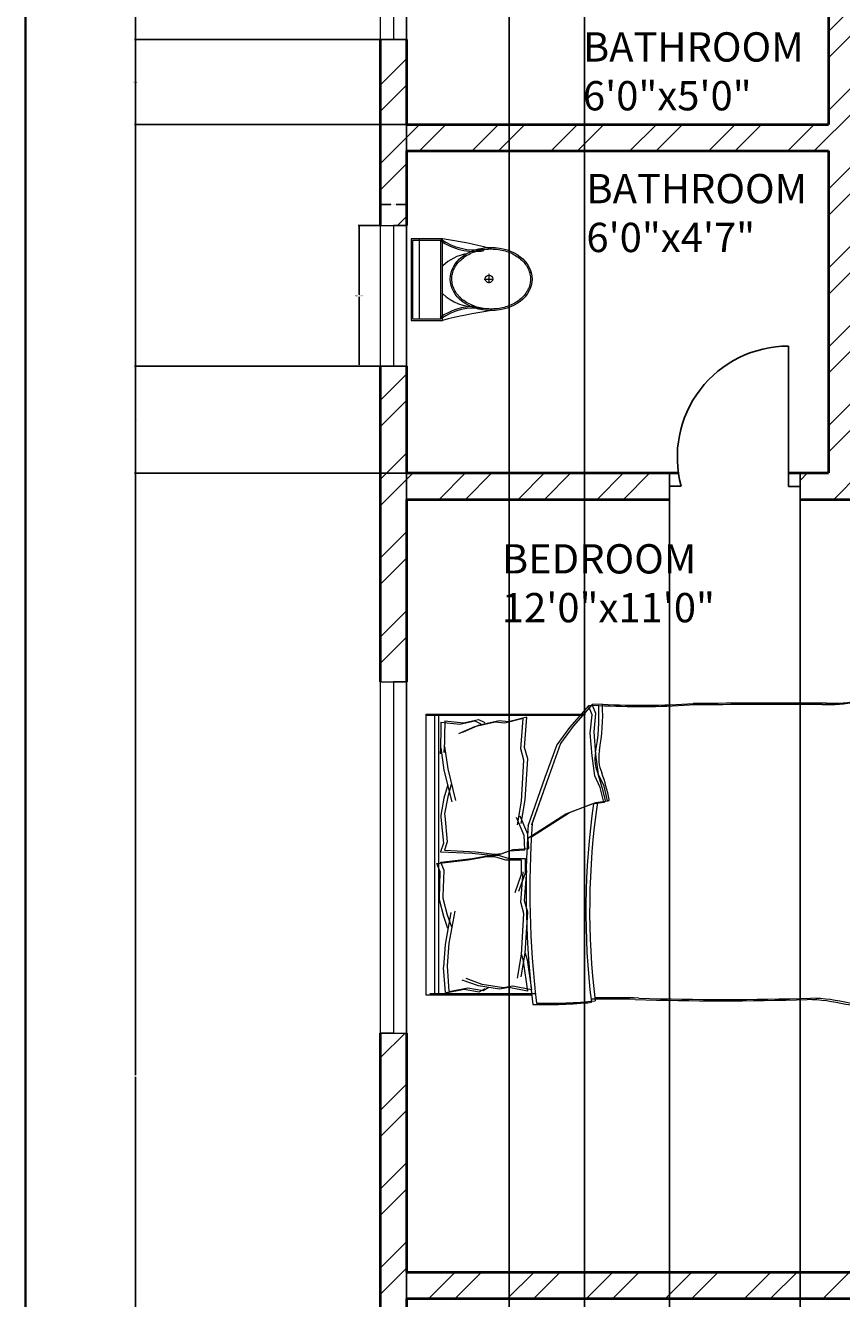
# Model space of a CAD drawing. Units: inches. Extents: x 2063 to 2617, y 1299 to 2210.
# Tile 6 of 22: x 2063 to 2202, y 1727 to 1945. Entities that reach past the tile are written whole.
import ezdxf

# ---------------------------------------------------------------- set-up
doc = ezdxf.new("R2010")
doc.units = ezdxf.units.IN
for name, color, linetype, lineweight in [('A-ANNO-DIMS', 2, 'Continuous', 18), ('A-ANNO-TTLB', 7, 'Continuous', 35), ('A-AREA-IDEN', 7, 'Continuous', 18), ('A-DOOR', 11, 'Continuous', 25), ('A-FLOR-FIXT', 8, 'Continuous', 18), ('A-FURN', 8, 'Continuous', 18), ('A-GLAZ', 123, 'Continuous', 18), ('A-WALL', 7, 'Continuous', 40)]:
    doc.layers.add(name, color=color, linetype=linetype, lineweight=lineweight)
doc.layers.add('A-WALL-PATT', color=215, linetype='Continuous', lineweight=13, true_color=0xa953a0)
doc.styles.get("Standard").update_dxf_attribs({"font": 'arial.ttf'})
doc.dimstyles.get("Standard").update_dxf_attribs({"dimtxt": 0.18, "dimasz": 0.18, "dimexe": 0.18, "dimexo": 0.0625, "dimgap": 0.09, "dimtad": 0, "dimtih": 1, "dimtoh": 1, "dimdec": 4, "dimzin": 0, "dimdsep": 46, "dimtxsty": 'Standard', "dimcen": 0.09, "dimadec": 0, "dimazin": 0, "dimtfac": 1, "dimtdec": 4, "dimtofl": 0, "dimtmove": 0, "dimatfit": 3, "dimfxl": 1, "dimtolj": 1, "dimtzin": 0, "dimarcsym": 0})

# ---------------------------------------------------------------- blocks, each defined once
blk = doc.blocks.new('A$C31115884')
for p, q in [((283.1, 497.7), (223.4, 497.7)), ((257.5, 466.4), (257.5, 523.2)), ((0, 200), (0, 0)), ((520, 200), (0, 200)), ((10, 190), (10, 10)), ((510, 190), (10, 190)), ((510, 10), (510, 190)), ((520, 0), (520, 200)), ((510, 54.5), (0, 54.5)), ((10, 10), (510, 10)), ((0, 0), (520, 0))]:
    blk.add_line(p, q)
blk.add_circle((255.6, 496.4), 23.6)
for centre, radius, start, end in [((2777.7, -204.6), 2807, 165.4549, 171.71327), ((3237, 905), 2807, 188.28673, 194.5451), ((-294.5, 403.3), 364.7, 324.20913, 9.34987), ((-294.5, 403.3), 374.7, 324.20913, 9.34987), ((139.5, 406.2), 293.5, 315.84364, 2.65635), ((805.8, 403.3), 374.7, 179.20365, 215.79087), ((805.8, 403.3), 364.7, 170.65013, 215.79087), ((383.6, 406.2), 293.5, 190.27735, 224.15636)]:
    blk.add_arc(centre, radius, start, end)
blk.add_ellipse((256.2, 509.9), major_axis=(0, -260.7), ratio=0.772727)
blk.add_open_spline([(256.2, 259.2), (263.1, 259.2), (270, 259.7), (287.8, 262.3), (298.7, 265.1), (319.9, 273.1), (330.2, 278.4), (350.1, 291.1), (359.7, 298.7), (377.7, 315.9), (386.2, 325.5), (401.7, 346.6), (408.8, 358.1), (421.3, 382.5), (426.8, 395.5), (435.9, 422.4), (439.5, 436.4), (444.8, 465.1), (446.5, 479.7), (447.9, 509.2), (447.6, 524), (445, 553.3), (442.7, 567.8), (436.3, 596), (432.1, 609.7), (421.9, 636), (416, 648.6), (402.5, 672.1), (395, 683), (378.6, 703), (369.8, 712.1), (351.1, 728), (341.3, 734.8), (320.9, 746.2), (310.4, 750.7), (288.9, 757.3), (278, 759.4), (256, 761), (245, 760.6), (223.1, 757.2), (212.3, 754.3), (191.1, 746.1), (180.8, 740.7), (160.9, 727.8), (151.4, 720.1), (133.5, 702.7), (125.1, 693), (109.6, 671.7), (102.6, 660.2), (90.2, 635.7), (84.9, 622.7), (76, 595.6), (72.4, 581.6), (67.2, 552.9), (65.6, 538.2), (64.4, 508.8), (64.8, 494), (67.5, 464.7), (69.9, 450.2), (76.6, 422), (80.8, 408.3), (91.1, 382.2), (97.2, 369.7), (110.8, 346.3), (118.4, 335.4), (134.8, 315.6), (143.7, 306.7), (162.4, 290.9), (172.3, 284.2), (192.8, 273), (203.3, 268.6), (224.8, 262.2), (235.8, 260.2), (249.9, 259.3), (253, 259.2), (256.2, 259.2)], degree=3, knots=[0, 0, 0, 0, 0.110105, 0.110105, 0.285049, 0.285049, 0.459994, 0.459994, 0.634938, 0.634938, 0.809882, 0.809882, 0.984827, 0.984827, 1.159771, 1.159771, 1.334715, 1.334715, 1.50966, 1.50966, 1.684604, 1.684604, 1.859549, 1.859549, 2.034493, 2.034493, 2.209437, 2.209437, 2.384382, 2.384382, 2.559326, 2.559326, 2.73427, 2.73427, 2.909215, 2.909215, 3.084159, 3.084159, 3.259103, 3.259103, 3.434048, 3.434048, 3.608992, 3.608992, 3.783936, 3.783936, 3.958881, 3.958881, 4.133825, 4.133825, 4.30877, 4.30877, 4.483714, 4.483714, 4.658658, 4.658658, 4.833603, 4.833603, 5.008547, 5.008547, 5.183491, 5.183491, 5.358436, 5.358436, 5.53338, 5.53338, 5.708324, 5.708324, 5.883269, 5.883269, 6.058213, 6.058213, 6.233158, 6.233158, 6.283185, 6.283185, 6.283185, 6.283185])
blk = doc.blocks.new('BED-DOUBLE')
for p, q in [((3.48, 63.33), (3.48, 81.44)), ((3.48, 63.33), (3.48, 81.44)), ((3.48, 81.44), (51.49, 81.44)), ((3.7, 62.69), (3.7, 80.8)), ((3.7, 62.69), (3.7, 80.8)), ((51.27, 81.44), (51.27, 54.83)), ((51.27, 81.44), (51.27, 54.83)), ((51.49, 81.44), (51.49, 80.8)), ((51.49, 80.8), (51.49, 54.19)), ((51.49, 80.8), (51.49, 54.19)), ((3.48, 79.91), (51.27, 79.91)), ((3.48, 79.91), (51.27, 79.91)), ((3.7, 79.27), (51.49, 79.27)), ((3.7, 79.27), (51.49, 79.27)), ((3.9, 78.11), (8.18, 78.43)), ((3.9, 78.11), (8.18, 78.43)), ((8.18, 78.43), (8.29, 78.42)), ((8.18, 78.43), (8.29, 78.42)), ((8.29, 78.42), (12.11, 78.13)), ((8.29, 78.42), (12.11, 78.13)), ((14.86, 77.69), (16.88, 78.42)), ((14.86, 77.69), (16.88, 78.42)), ((16.88, 78.42), (19.77, 79.14)), ((16.88, 78.42), (19.77, 79.14)), ((17.11, 77.78), (20, 78.5)), ((17.11, 77.78), (20, 78.5)), ((19.77, 79.14), (20.09, 79.14)), ((19.77, 79.14), (20.09, 79.14)), ((20, 78.5), (20.32, 78.5)), ((20, 78.5), (20.32, 78.5)), ((20.09, 79.14), (24.54, 79)), ((20.09, 79.14), (24.54, 79)), ((20.32, 78.5), (24.77, 78.36)), ((20.32, 78.5), (24.77, 78.36)), ((24.54, 79), (25.98, 79.57)), ((24.54, 79), (25.98, 79.57)), ((24.77, 78.36), (26.21, 78.93)), ((24.77, 78.36), (26.21, 78.93)), ((25.98, 79.57), (26.56, 74.22)), ((25.98, 79.57), (26.56, 74.22)), ((26.21, 78.93), (26.79, 73.58)), ((26.21, 78.93), (26.79, 73.58)), ((27.98, 78.95), (27.73, 73.58)), ((27.98, 78.95), (27.73, 73.58)), ((28.21, 78.31), (27.96, 72.94)), ((28.21, 78.31), (27.96, 72.94)), ((29.46, 78.46), (27.98, 78.95)), ((29.46, 78.46), (27.98, 78.95)), ((29.68, 77.83), (28.21, 78.31)), ((29.68, 77.83), (28.21, 78.31)), ((33.88, 78.89), (29.46, 78.46)), ((33.88, 78.89), (29.46, 78.46)), ((34.21, 78.91), (33.88, 78.89)), ((34.2, 78.91), (33.88, 78.89)), ((37.14, 78.37), (34.2, 78.91)), ((37.14, 78.37), (34.21, 78.91)), ((41.91, 78.37), (36.5, 77.02)), ((41.91, 78.37), (36.5, 77.02)), ((39.2, 77.77), (37.14, 78.37)), ((39.2, 77.77), (37.14, 78.37)), ((45.71, 78.9), (41.91, 78.37)), ((45.71, 78.9), (41.91, 78.37)), ((50.11, 78.89), (44.71, 78.98)), ((44.71, 78.98), (45.71, 78.9)), ((50.11, 78.89), (44.71, 78.98)), ((44.71, 78.98), (45.71, 78.9)), ((50.34, 78.25), (44.94, 78.34)), ((44.94, 78.34), (45.94, 78.26)), ((50.34, 78.25), (44.94, 78.34)), ((44.94, 78.34), (45.94, 78.26)), ((50.11, 78.89), (49.73, 75.68)), ((50.11, 78.89), (49.73, 75.68)), ((3.89, 78.13), (4.47, 74.95)), ((3.9, 78.13), (4.47, 74.95)), ((4.12, 77.49), (4.7, 74.31)), ((4.12, 77.49), (4.7, 74.31)), ((4.13, 77.47), (8.41, 77.8)), ((4.13, 77.47), (8.41, 77.8)), ((8.41, 77.8), (8.51, 77.78)), ((8.41, 77.8), (8.51, 77.78)), ((8.51, 77.78), (12.34, 77.49)), ((8.51, 77.78), (12.34, 77.49)), ((12.11, 78.13), (17.6, 77.12)), ((12.11, 78.13), (17.6, 77.12)), ((12.34, 77.49), (17.83, 76.48)), ((12.34, 77.49), (17.83, 76.48)), ((15.08, 77.05), (17.11, 77.78)), ((15.08, 77.05), (17.11, 77.78)), ((34.11, 78.25), (29.68, 77.83)), ((34.11, 78.25), (29.68, 77.83)), ((34.43, 78.27), (34.11, 78.25)), ((34.43, 78.27), (34.11, 78.25)), ((37.36, 77.73), (34.43, 78.27)), ((37.36, 77.73), (34.43, 78.27)), ((42.14, 77.73), (36.72, 76.38)), ((42.14, 77.73), (36.72, 76.38)), ((39.43, 77.13), (37.36, 77.73)), ((39.43, 77.13), (37.36, 77.73)), ((45.94, 78.26), (42.14, 77.73)), ((45.94, 78.26), (42.14, 77.73)), ((50.34, 78.25), (49.96, 75.04)), ((50.34, 78.25), (49.96, 75.04)), ((4.47, 74.95), (4.04, 72.34)), ((4.47, 74.95), (4.04, 72.34)), ((4.7, 74.31), (4.27, 71.7)), ((4.7, 74.31), (4.27, 71.7)), ((5.05, 72.49), (6.06, 75.24)), ((5.05, 72.49), (6.06, 75.24)), ((5.28, 71.85), (6.29, 74.6)), ((5.28, 71.85), (6.29, 74.6)), ((26.56, 74.22), (27.14, 71.04)), ((26.56, 74.22), (27.14, 71.04)), ((49.31, 73.19), (48.13, 75.87)), ((49.31, 73.19), (48.13, 75.87)), ((49.54, 72.55), (48.36, 75.23)), ((49.54, 72.55), (48.36, 75.23)), ((49.73, 75.68), (50.33, 73.11)), ((49.73, 75.68), (50.33, 73.11)), ((49.96, 75.04), (50.56, 72.47)), ((49.96, 75.04), (50.56, 72.47)), ((4.04, 72.34), (4.62, 71.33)), ((4.04, 72.34), (4.62, 71.33)), ((4.47, 68.87), (5.05, 72.49)), ((4.47, 68.87), (5.05, 72.49)), ((4.7, 68.23), (5.28, 71.85)), ((4.7, 68.23), (5.28, 71.85)), ((26.79, 73.58), (27.37, 70.4)), ((26.79, 73.58), (27.37, 70.4)), ((27.73, 73.58), (27.36, 70.37)), ((27.73, 73.58), (27.36, 70.37)), ((27.96, 72.94), (27.58, 69.73)), ((27.96, 72.94), (27.58, 69.73)), ((50.11, 69.61), (49.31, 73.19)), ((50.11, 69.61), (49.31, 73.19)), ((50.34, 68.98), (49.54, 72.55)), ((50.34, 68.98), (49.54, 72.55)), ((50.33, 73.11), (49.81, 72.06)), ((50.33, 73.11), (49.82, 72.06)), ((50.56, 72.47), (50.04, 71.42)), ((50.56, 72.47), (50.04, 71.42)), ((4.27, 71.7), (4.85, 70.69)), ((4.27, 71.7), (4.85, 70.69)), ((27.14, 69.74), (26.56, 67.86)), ((27.14, 69.74), (26.56, 67.86)), ((27.14, 71.04), (27.14, 69.74)), ((27.14, 71.04), (27.14, 69.74)), ((27.36, 70.37), (27.44, 69.07)), ((27.36, 70.37), (27.44, 69.07)), ((27.37, 70.4), (27.37, 69.1)), ((27.37, 70.4), (27.37, 69.1)), ((27.58, 69.73), (27.66, 68.43)), ((27.58, 69.73), (27.66, 68.43)), ((49.92, 68.01), (50.11, 69.61)), ((49.92, 68.01), (50.11, 69.61)), ((4.76, 67.28), (4.47, 68.87)), ((4.76, 67.28), (4.47, 68.87)), ((4.99, 66.64), (4.7, 68.23)), ((4.99, 66.64), (4.7, 68.23)), ((26.56, 67.86), (26.56, 65.18)), ((26.56, 67.86), (26.56, 65.18)), ((27.37, 69.1), (26.79, 67.22)), ((27.37, 69.1), (26.79, 67.22)), ((27.44, 69.07), (28.13, 67.23)), ((27.44, 69.07), (28.13, 67.23)), ((27.66, 68.43), (28.36, 66.59)), ((27.66, 68.43), (28.36, 66.59)), ((50.7, 64.87), (49.92, 68.01)), ((50.7, 64.87), (49.92, 68.01)), ((50.15, 67.37), (50.34, 68.98)), ((50.15, 67.37), (50.34, 68.98)), ((4.18, 64.1), (4.76, 67.28)), ((4.18, 64.1), (4.76, 67.28)), ((4.41, 63.46), (4.99, 66.64)), ((4.41, 63.46), (4.99, 66.64)), ((6.38, 65.82), (10.41, 65.15)), ((6.38, 65.82), (10.41, 65.15)), ((17.42, 64.72), (19.38, 65.27)), ((17.42, 64.72), (19.38, 65.27)), ((19.38, 65.27), (24.52, 64.87)), ((19.38, 65.27), (24.52, 64.87)), ((24.1, 65.18), (20.96, 66.27)), ((24.1, 65.18), (20.96, 66.27)), ((24.33, 64.54), (21.19, 65.63)), ((24.33, 64.54), (21.19, 65.63)), ((26.79, 67.22), (26.79, 64.54)), ((26.79, 67.22), (26.79, 64.54)), ((28.13, 67.23), (28.3, 64.55)), ((28.13, 67.23), (28.3, 64.55)), ((28.36, 66.59), (28.53, 63.91)), ((28.36, 66.59), (28.53, 63.91)), ((30.75, 64.7), (33.82, 65.99)), ((30.75, 64.7), (33.82, 65.99)), ((30.98, 64.06), (34.05, 65.35)), ((30.98, 64.06), (34.05, 65.35)), ((32.56, 65.82), (36.6, 65.15)), ((32.56, 65.82), (36.6, 65.15)), ((43.61, 64.72), (45.57, 65.27)), ((43.61, 64.72), (45.57, 65.27)), ((45.57, 65.27), (50.7, 64.87)), ((45.57, 65.27), (50.7, 64.87)), ((50.93, 64.23), (50.15, 67.37)), ((50.93, 64.23), (50.15, 67.37)), ((9.28, 64.83), (4.18, 64.1)), ((9.28, 64.83), (4.18, 64.1)), ((9.51, 64.19), (4.41, 63.46)), ((9.51, 64.19), (4.41, 63.46)), ((6.61, 65.18), (10.64, 64.51)), ((6.61, 65.18), (10.64, 64.51)), ((10.41, 65.15), (9.28, 64.83)), ((10.41, 65.15), (9.28, 64.83)), ((10.64, 64.51), (9.51, 64.19)), ((10.64, 64.51), (9.51, 64.19)), ((10.41, 65.15), (17.42, 64.72)), ((10.41, 65.15), (17.42, 64.72)), ((10.64, 64.51), (17.65, 64.08)), ((10.64, 64.51), (17.65, 64.08)), ((17.65, 64.08), (19.61, 64.64)), ((17.65, 64.08), (19.61, 64.64)), ((19.61, 64.64), (24.74, 64.23)), ((19.61, 64.64), (24.74, 64.23)), ((26.56, 65.18), (24.1, 65.18)), ((26.56, 65.18), (24.1, 65.18)), ((26.79, 64.54), (24.33, 64.54)), ((26.79, 64.54), (24.33, 64.54)), ((28.3, 64.55), (30.75, 64.7)), ((28.3, 64.55), (30.75, 64.7)), ((28.53, 63.91), (30.98, 64.06)), ((28.53, 63.91), (30.98, 64.06)), ((30.26, 64.06), (34.45, 57.57)), ((30.26, 64.06), (34.45, 57.57)), ((30.49, 63.42), (34.68, 56.93)), ((30.49, 63.42), (34.68, 56.93)), ((40.64, 61.13), (32.31, 64.06)), ((40.64, 61.13), (32.31, 64.06)), ((40.87, 60.49), (32.53, 63.42)), ((40.87, 60.49), (32.54, 63.42)), ((32.79, 65.18), (36.83, 64.51)), ((32.79, 65.18), (36.82, 64.51)), ((36.6, 65.15), (43.61, 64.72)), ((36.6, 65.15), (43.61, 64.72)), ((36.82, 64.51), (43.83, 64.08)), ((36.83, 64.51), (43.84, 64.08)), ((43.83, 64.08), (45.8, 64.64)), ((43.84, 64.08), (45.8, 64.64)), ((45.8, 64.64), (50.93, 64.23)), ((45.8, 64.64), (50.93, 64.23)), ((46.22, 59.11), (40.64, 61.13)), ((46.22, 59.11), (40.64, 61.13)), ((46.45, 58.48), (40.87, 60.49)), ((46.45, 58.48), (40.87, 60.49)), ((49.16, 56.95), (46.22, 59.11)), ((49.16, 56.95), (46.22, 59.11)), ((34.45, 57.57), (36.15, 53.08)), ((34.45, 57.57), (36.15, 53.08)), ((34.68, 56.93), (36.38, 52.44)), ((34.68, 56.93), (36.38, 52.44)), ((49.39, 56.31), (46.45, 58.48)), ((49.39, 56.31), (46.45, 58.48)), ((52.87, 53.7), (49.16, 56.95)), ((52.87, 53.7), (49.16, 56.95)), ((53.1, 53.06), (49.39, 56.31)), ((53.1, 53.06), (49.39, 56.31)), ((36.15, 53.08), (36.46, 51.07)), ((36.15, 53.08), (36.46, 51.07)), ((36.38, 52.44), (36.69, 50.43)), ((36.38, 52.44), (36.69, 50.43)), ((38.94, 51.69), (40.95, 52.61)), ((38.94, 51.69), (40.95, 52.61)), ((40.95, 52.61), (44.36, 53.08)), ((40.95, 52.61), (44.36, 53.08)), ((41.18, 51.97), (44.59, 52.44)), ((41.18, 51.97), (44.59, 52.44)), ((44.36, 53.08), (48.23, 53.39)), ((44.36, 53.08), (48.23, 53.39)), ((44.59, 52.44), (48.46, 52.75)), ((44.59, 52.44), (48.46, 52.75)), ((48.23, 53.39), (51.33, 53.08)), ((48.23, 53.39), (51.33, 53.08)), ((48.46, 52.75), (51.56, 52.44)), ((48.46, 52.75), (51.56, 52.44)), ((51.33, 53.08), (52.87, 53.7)), ((51.33, 53.08), (52.87, 53.7)), ((51.56, 52.44), (53.1, 53.06)), ((51.56, 52.44), (53.1, 53.06)), ((52.95, 51.95), (52.87, 53.7, 3.87)), ((52.95, 51.95), (52.87, 53.7, 3.87)), ((53.18, 51.31), (53.1, 53.06, 3.87)), ((53.18, 51.31), (53.1, 53.06, 3.87)), ((36.46, 51.07), (38.94, 51.69)), ((36.46, 51.07), (38.94, 51.69)), ((36.69, 50.43), (39.17, 51.05)), ((36.69, 50.43), (39.17, 51.05)), ((39.17, 51.05), (41.18, 51.97)), ((39.17, 51.05), (41.18, 51.97)), ((15.06, 2.2), (39.68, 2.2)), ((15.06, 2.2), (39.68, 2.2)), ((15.29, 1.56), (39.91, 1.56)), ((15.29, 1.56), (39.91, 1.56))]:
    blk.add_line(p, q)
for centre, radius, start, end in [((85.16, 61.35), 83.31, 178.7218, 185.604), ((85.16, 61.35), 83.31, 178.7218, 185.604), ((21.36, -100.61), 164.97, 86.0865, 96.7821), ((21.36, -100.61), 164.97, 86.0865, 96.7821), ((21.59, -101.25), 164.97, 86.0865, 96.7821), ((21.59, -101.25), 164.97, 86.0865, 96.7821), ((85.39, 60.71), 83.31, 178.7218, 185.604), ((85.39, 60.71), 83.31, 178.7218, 185.604), ((17.76, -74.87), 129.02, 81.7845, 96.9006), ((17.76, -74.87), 129.02, 81.7845, 96.9006), ((17.98, -75.51), 129.02, 81.7845, 96.9006), ((17.98, -75.51), 129.02, 81.7845, 96.9006), ((-167.31, 50.27), 170.11, 358.4762, 1.0082), ((-167.31, 50.27), 170.11, 358.4762, 1.0082), ((-167.08, 49.63), 170.11, 358.4762, 1.0082), ((-167.08, 49.63), 170.11, 358.4762, 1.0082), ((43.74, 46.38), 6.22, 78.6608, 113.7384), ((43.74, 46.38), 6.22, 78.6608, 113.7384), ((51.33, 88.1), 36.18, 259.8763, 272.5657), ((51.33, 88.1), 36.18, 259.8763, 272.5657), ((36.64, 51), 0.185, 160.2464, 271.1377), ((36.64, 51), 0.185, 160.2464, 271.1377), ((31.15, 79.96), 29.65, 280.6617, 289.8806), ((31.15, 79.96), 29.65, 280.6617, 289.8806), ((36.87, 50.36), 0.185, 160.2464, 271.1377), ((36.86, 50.36), 0.185, 160.2464, 271.1377), ((31.38, 79.32), 29.65, 280.6617, 289.8806), ((31.38, 79.32), 29.65, 280.6617, 289.8806), ((43.97, 45.74), 6.22, 78.6608, 113.7384), ((43.97, 45.74), 6.22, 78.6608, 113.7384), ((51.56, 87.46), 36.18, 259.8763, 272.5657), ((51.56, 87.46), 36.18, 259.8763, 272.5657), ((182.27, 45.13), 129.5, 176.9791, 183.8365), ((182.27, 45.13), 129.5, 176.9791, 183.8365), ((182.49, 44.49), 129.5, 176.9791, 183.8365), ((182.49, 44.49), 129.5, 176.9791, 183.8365), ((484.82, 30.83), 482.31, 178.2277, 181.7185), ((484.82, 30.83), 482.31, 178.2277, 181.7185), ((485.05, 30.19), 482.31, 178.2277, 181.7185), ((485.05, 30.19), 482.31, 178.2277, 181.7185), ((-4508.74, 13.62), 4561.86, 0.00217, 0.28689), ((-4508.74, 13.62), 4561.86, 0.00217, 0.28689), ((-4508.51, 12.98), 4561.86, 0.00217, 0.28689), ((-4508.51, 12.98), 4561.86, 0.00217, 0.28689), ((-26.9, 16.93), 29.63, 346.0648, 358.9113), ((-26.9, 16.93), 29.63, 346.0648, 358.9113), ((-26.67, 16.29), 29.63, 346.0648, 358.9113), ((-26.67, 16.29), 29.63, 346.0648, 358.9113), ((76.16, 12.78), 23.07, 177.4714, 206.4681), ((76.16, 12.78), 23.07, 177.4714, 206.4681), ((76.39, 12.14), 23.07, 177.4714, 206.4681), ((76.39, 12.14), 23.07, 177.4714, 206.4681), ((-21.66, 11.17), 23.56, 337.9751, 356.652), ((-21.66, 11.17), 23.56, 337.9751, 356.652), ((-21.43, 10.53), 23.56, 337.9751, 356.652), ((-21.43, 10.53), 23.56, 337.9751, 356.652), ((1.09, 1.73), 1.09, 146.1736, 293.4781), ((1.09, 1.73), 1.09, 146.1736, 293.4781), ((21.43, -119.39), 121.76, 92.9958, 99.4091), ((21.43, -119.39), 121.76, 92.9958, 99.4091), ((-17.22, 105.16), 106.46, 283.3832, 287.7053), ((-17.22, 105.16), 106.46, 283.3832, 287.7053), ((-16.99, 104.52), 106.46, 283.3832, 287.7053), ((-16.99, 104.52), 106.46, 283.3832, 287.7053), ((41.15, -130.83), 133.04, 84.4998, 90.6351), ((41.15, -130.83), 133.04, 84.4998, 90.6351), ((54.41, 2.57), 1.1, 242.6588, 356.02), ((54.41, 2.57), 1.1, 242.6588, 356.02), ((1.32, 1.09), 1.09, 146.1736, 293.4781), ((1.32, 1.09), 1.09, 146.1736, 293.4781), ((21.66, -120.03), 121.76, 92.9958, 99.4091), ((21.66, -120.03), 121.76, 92.9958, 99.4091), ((41.38, -131.47), 133.04, 84.4998, 90.6351), ((41.38, -131.47), 133.04, 84.4998, 90.6351), ((54.64, 1.93), 1.1, 242.6588, 356.02), ((54.64, 1.93), 1.1, 242.6588, 356.02)]:
    blk.add_arc(centre, radius, start, end)
blk = doc.blocks.new('WIN-60IN')
for p, q in [((0, 60), (4.5, 60)), ((0, 60), (0, 0)), ((4.5, 60), (2.25, 60)), ((2.25, 60), (2.25, 0)), ((4.5, 60), (4.5, 0)), ((2.25, 0), (0, 0)), ((0, 0), (4.5, 0))]:
    blk.add_line(p, q)
blk = doc.blocks.new('WIN-24IN')
for p, q in [((0, 24), (4.5, 24)), ((0, 24), (0, 0)), ((4.5, 24), (2.25, 24)), ((2.25, 24), (2.25, 0)), ((4.5, 24), (4.5, 0)), ((2.25, 0), (0, 0)), ((0, 0), (4.5, 0))]:
    blk.add_line(p, q)
blk = doc.blocks.new('*D17')
at = {"layer": 'A-ANNO-DIMS', "color": 0, "lineweight": -2, "transparency": 16777216}
for p, q in [((2123.08, 1910.58), (2119.36, 1910.58)), ((2119.54, 1910.4), (2119.54, 1898.76)), ((2119.54, 1886.76), (2119.54, 1898.4)), ((2123.08, 1886.58), (2119.36, 1886.58))]:
    blk.add_line(p, q, dxfattribs=at)
at = {"layer": 'A-ANNO-DIMS', "color": 0, "transparency": 16777216}
for points in [[(2119.51, 1910.4), (2119.57, 1910.4), (2119.54, 1910.58)], [(2119.51, 1886.76), (2119.57, 1886.76), (2119.54, 1886.58)]]:
    blk.add_solid(points, dxfattribs=at)
at = {"layer": 'Defpoints', "color": 0, "transparency": 16777216}
for p in [(2119.54, 1910.58), (2123.14, 1910.58), (2123.14, 1886.58)]:
    blk.add_point(p, dxfattribs=at)
at = {"layer": 'A-ANNO-DIMS', "color": 0, "transparency": 16777216, "insert": (2119.54, 1898.58), "char_height": 0.18, "attachment_point": 5}
blk.add_mtext('\\A1;WIN. 24 TYP.', dxfattribs=at)
blk = doc.blocks.new('*D18')
at = {"layer": 'A-ANNO-DIMS', "color": 0, "lineweight": -2, "transparency": 16777216}
for p, q in [((2123.14, 1910.65), (2123.14, 1914.36)), ((2123.32, 1914.18), (2124.94, 1914.18)), ((2127.46, 1914.18), (2125.85, 1914.18)), ((2127.64, 1910.65), (2127.64, 1914.36))]:
    blk.add_line(p, q, dxfattribs=at)
at = {"layer": 'A-ANNO-DIMS', "color": 0, "transparency": 16777216}
for points in [[(2123.32, 1914.21), (2123.32, 1914.15), (2123.14, 1914.18)], [(2127.46, 1914.21), (2127.46, 1914.15), (2127.64, 1914.18)]]:
    blk.add_solid(points, dxfattribs=at)
at = {"layer": 'Defpoints', "color": 0, "transparency": 16777216}
for p in [(2127.64, 1914.18), (2123.14, 1910.58), (2127.64, 1910.58)]:
    blk.add_point(p, dxfattribs=at)
at = {"layer": 'A-ANNO-DIMS', "color": 0, "transparency": 16777216, "insert": (2125.39, 1914.18), "char_height": 0.18, "attachment_point": 5}
blk.add_mtext('\\A1;5 TYP.', dxfattribs=at)
blk = doc.blocks.new('*D32')
at = {"layer": 'A-ANNO-DIMS', "color": 0, "lineweight": -2, "transparency": 16777216}
for p, q in [((2123.08, 2128.81), (2081.21, 2128.81)), ((2081.39, 2128.63), (2081.39, 1765.49)), ((2081.39, 1401.99), (2081.39, 1765.13)), ((2123.08, 1401.81), (2081.21, 1401.81))]:
    blk.add_line(p, q, dxfattribs=at)
at = {"layer": 'A-ANNO-DIMS', "color": 0, "transparency": 16777216}
for points in [[(2081.36, 2128.63), (2081.42, 2128.63), (2081.39, 2128.81)], [(2081.36, 1401.99), (2081.42, 1401.99), (2081.39, 1401.81)]]:
    blk.add_solid(points, dxfattribs=at)
at = {"layer": 'Defpoints', "color": 0, "transparency": 16777216}
for p in [(2081.39, 2128.81), (2123.14, 2128.81), (2123.14, 1401.81)]:
    blk.add_point(p, dxfattribs=at)
at = {"layer": 'A-ANNO-DIMS', "color": 0, "transparency": 16777216, "insert": (2081.39, 1765.31), "char_height": 0.18, "attachment_point": 5}
blk.add_mtext('\\A1;727', dxfattribs=at)
blk = doc.blocks.new('*D49')
at = {"layer": 'A-ANNO-DIMS', "color": 0, "lineweight": -2, "transparency": 16777216}
for p, q in [((2127.64, 2124.25), (2127.64, 1317.7)), ((2158.04, 2124.25), (2158.04, 1317.7)), ((2127.82, 1317.88), (2142.38, 1317.88)), ((2157.86, 1317.88), (2143.31, 1317.88))]:
    blk.add_line(p, q, dxfattribs=at)
at = {"layer": 'A-ANNO-DIMS', "color": 0, "transparency": 16777216}
for points in [[(2127.82, 1317.91), (2127.82, 1317.85), (2127.64, 1317.88)], [(2157.86, 1317.91), (2157.86, 1317.85), (2158.04, 1317.88)]]:
    blk.add_solid(points, dxfattribs=at)
at = {"layer": 'Defpoints', "color": 0, "transparency": 16777216}
for p in [(2127.64, 2124.31), (2158.04, 2124.31), (2158.04, 1317.88)]:
    blk.add_point(p, dxfattribs=at)
at = {"layer": 'A-ANNO-DIMS', "color": 0, "transparency": 16777216, "insert": (2142.84, 1317.88), "char_height": 0.18, "attachment_point": 5}
blk.add_mtext('\\A1;30.396', dxfattribs=at)
blk = doc.blocks.new('*D57')
at = {"layer": 'A-ANNO-DIMS', "color": 0, "lineweight": -2, "transparency": 16777216}
for p, q in [((2172.52, 1868.25), (2172.52, 1317.7)), ((2194.82, 1868.25), (2194.82, 1317.7)), ((2172.7, 1317.88), (2183.2, 1317.88)), ((2194.64, 1317.88), (2184.14, 1317.88))]:
    blk.add_line(p, q, dxfattribs=at)
at = {"layer": 'A-ANNO-DIMS', "color": 0, "transparency": 16777216}
for points in [[(2172.7, 1317.91), (2172.7, 1317.85), (2172.52, 1317.88)], [(2194.64, 1317.91), (2194.64, 1317.85), (2194.82, 1317.88)]]:
    blk.add_solid(points, dxfattribs=at)
at = {"layer": 'Defpoints', "color": 0, "transparency": 16777216}
for p in [(2172.52, 1868.31), (2194.82, 1868.31), (2194.82, 1317.88)]:
    blk.add_point(p, dxfattribs=at)
at = {"layer": 'A-ANNO-DIMS', "color": 0, "transparency": 16777216, "insert": (2183.67, 1317.88), "char_height": 0.18, "attachment_point": 5}
blk.add_mtext('\\A1;22.305', dxfattribs=at)
blk = doc.blocks.new('*D61')
at = {"layer": 'A-ANNO-DIMS', "color": 0, "lineweight": -2, "transparency": 16777216}
for p, q in [((2127.64, 1442.37), (2127.64, 2170.74)), ((2127.82, 2170.56), (2136.03, 2170.56)), ((2144.97, 2170.56), (2136.77, 2170.56)), ((2145.15, 1442.37), (2145.15, 2170.74))]:
    blk.add_line(p, q, dxfattribs=at)
at = {"layer": 'A-ANNO-DIMS', "color": 0, "transparency": 16777216}
for points in [[(2127.82, 2170.59), (2127.82, 2170.53), (2127.64, 2170.56)], [(2144.97, 2170.59), (2144.97, 2170.53), (2145.15, 2170.56)]]:
    blk.add_solid(points, dxfattribs=at)
at = {"layer": 'Defpoints', "color": 0, "transparency": 16777216}
for p in [(2145.15, 2170.56), (2127.64, 1442.31), (2145.15, 1442.31)]:
    blk.add_point(p, dxfattribs=at)
at = {"layer": 'A-ANNO-DIMS', "color": 0, "transparency": 16777216, "insert": (2136.4, 2170.56), "char_height": 0.18, "attachment_point": 5}
blk.add_mtext('\\A1;17.51', dxfattribs=at)
blk = doc.blocks.new('*D65')
at = {"layer": 'A-ANNO-DIMS', "color": 0, "lineweight": -2, "transparency": 16777216}
for p, q in [((2127.58, 1886.58), (2081.21, 1886.58)), ((2081.39, 1886.4), (2081.39, 1877.63)), ((2081.39, 1868.49), (2081.39, 1877.27)), ((2127.58, 1868.31), (2081.21, 1868.31))]:
    blk.add_line(p, q, dxfattribs=at)
at = {"layer": 'A-ANNO-DIMS', "color": 0, "transparency": 16777216}
for points in [[(2081.36, 1886.4), (2081.42, 1886.4), (2081.39, 1886.58)], [(2081.36, 1868.49), (2081.42, 1868.49), (2081.39, 1868.31)]]:
    blk.add_solid(points, dxfattribs=at)
at = {"layer": 'Defpoints', "color": 0, "transparency": 16777216}
for p in [(2081.39, 1886.58), (2127.64, 1886.58), (2127.64, 1868.31)]:
    blk.add_point(p, dxfattribs=at)
at = {"layer": 'A-ANNO-DIMS', "color": 0, "transparency": 16777216, "insert": (2081.39, 1877.45), "char_height": 0.18, "attachment_point": 5}
blk.add_mtext('\\A1;18.27', dxfattribs=at)
blk = doc.blocks.new('*D66')
at = {"layer": 'A-ANNO-DIMS', "color": 0, "lineweight": -2, "transparency": 16777216}
for p, q in [((2127.58, 1942.35), (2081.21, 1942.35)), ((2081.39, 1942.17), (2081.39, 1935.26)), ((2081.39, 1927.99), (2081.39, 1934.9)), ((2127.58, 1927.81), (2081.21, 1927.81))]:
    blk.add_line(p, q, dxfattribs=at)
at = {"layer": 'A-ANNO-DIMS', "color": 0, "transparency": 16777216}
for points in [[(2081.36, 1942.17), (2081.42, 1942.17), (2081.39, 1942.35)], [(2081.36, 1927.99), (2081.42, 1927.99), (2081.39, 1927.81)]]:
    blk.add_solid(points, dxfattribs=at)
at = {"layer": 'Defpoints', "color": 0, "transparency": 16777216}
for p in [(2081.39, 1942.35), (2127.64, 1942.35), (2127.64, 1927.81)]:
    blk.add_point(p, dxfattribs=at)
at = {"layer": 'A-ANNO-DIMS', "color": 0, "transparency": 16777216, "insert": (2081.39, 1935.08), "char_height": 0.18, "attachment_point": 5}
blk.add_mtext('\\A1;14.537', dxfattribs=at)

msp = doc.modelspace()

# ---------------------------------------------------------------- hatches: boundary and pattern name
at = {"layer": 'A-WALL-PATT'}
h = msp.add_hatch(dxfattribs=at)
h.set_pattern_fill('ANSI32', color=256)
h.paths.add_polyline_path([(2553.6442, 2128.8122), (2511.1703, 2128.8122), (2511.1703, 2124.3122), (2549.1442, 2124.3122), (2549.1442, 2095.662), (2553.6442, 2095.662)])
h.paths.add_polyline_path([(2553.6442, 2035.662), (2549.1442, 2035.662), (2549.1442, 1980.3122), (2503.7214, 1980.3122), (2503.7214, 1975.8122), (2549.1442, 1975.8122), (2549.1442, 1962.9693), (2553.6442, 1962.9693)])
h.paths.add_polyline_path([(2553.6442, 1938.9693), (2549.1442, 1938.9693), (2549.1442, 1927.8122), (2477.1442, 1927.8122), (2477.1442, 1975.8122), (2481.2918, 1975.8122), (2481.2918, 1980.3122), (2453.2648, 1980.3122), (2453.2648, 1975.8122), (2472.6442, 1975.8122), (2472.6442, 1868.3122), (2400.6442, 1868.3122), (2400.6442, 1861.3782), (2405.1442, 1861.3782), (2405.1442, 1863.8122), (2480.9699, 1863.8122), (2480.9699, 1866.0622), (2480.9699, 1868.3122), (2477.1442, 1868.3122), (2477.1442, 1923.3122), (2549.1442, 1923.3122), (2549.1442, 1908.8504), (2553.6442, 1908.8504)])
h.paths.add_polyline_path([(2553.6442, 1884.8504), (2549.1442, 1884.8504), (2549.1442, 1868.3122), (2501.0636, 1868.3122), (2501.0636, 1863.8122), (2549.1442, 1863.8122), (2549.1442, 1826.0298), (2553.6442, 1826.0298)])
h.paths.add_polyline_path([(2388.1504, 1980.3122), (2340.6442, 1980.3122), (2340.6442, 2124.3122), (2358.7501, 2124.3122), (2358.7501, 2128.8122), (2316.3482, 2128.8122), (2316.3482, 2124.3122), (2336.1442, 2124.3122), (2336.1442, 1980.3122), (2289.1737, 1980.3122), (2289.1737, 1975.8122), (2336.1442, 1975.8122), (2336.1442, 1619.3122), (2333.1433, 1619.3122), (2333.1433, 1614.8122), (2344.1671, 1614.8122), (2344.1671, 1617.0622), (2344.1671, 1619.3122), (2340.6442, 1619.3122), (2340.6442, 1975.8122), (2388.1504, 1975.8122), (2388.1504, 1978.0622)])
h.paths.add_polyline_path([(2290.1442, 1614.8122), (2301.4594, 1614.8122), (2301.4594, 1617.0622), (2301.4594, 1619.3122), (2285.6442, 1619.3122), (2285.6442, 1566.8122), (2280.8619, 1566.8122), (2280.8619, 1564.5622), (2280.8619, 1562.3122), (2285.6442, 1562.3122), (2285.6442, 1442.3122), (2281.7879, 1442.3122), (2281.7879, 1437.8122), (2285.6442, 1437.8122), (2285.6442, 1401.8122), (2290.1442, 1401.8122)])
h.paths.add_polyline_path([(2549.1442, 1731.8122), (2405.1442, 1731.8122), (2405.1442, 1834.4638), (2402.8942, 1834.4638), (2400.6442, 1834.4638), (2400.6442, 1727.3122), (2549.1442, 1727.3122)])
h.paths.add_polyline_path([(2553.6442, 1766.0298), (2551.3942, 1766.0298), (2549.1442, 1766.0298), (2549.1442, 1686.7767), (2553.6442, 1686.7767)])
h.paths.add_polyline_path([(2553.6442, 1638.7767), (2551.3942, 1638.7767), (2549.1442, 1638.7767), (2549.1442, 1619.3122), (2448.6442, 1619.3122), (2448.6442, 1610.5671), (2450.8942, 1610.5671), (2453.1442, 1610.5671), (2453.1442, 1614.8122), (2549.1442, 1614.8122), (2549.1442, 1601.6421), (2553.6442, 1601.6421)])
h.paths.add_polyline_path([(2553.6442, 1577.6421), (2551.3942, 1577.6421), (2549.1442, 1577.6421), (2549.1442, 1566.8122), (2453.1442, 1566.8122), (2453.1442, 1591.5045), (2451.0335, 1591.5045), (2448.6442, 1591.5045), (2448.6442, 1566.8122), (2434.0475, 1566.8122), (2434.0475, 1562.3122), (2549.1442, 1562.3122), (2549.1442, 1533.48), (2553.6442, 1533.48)])
h.paths.add_polyline_path([(2553.6442, 1473.48), (2549.1442, 1473.48), (2549.1442, 1442.3122), (2502.6258, 1442.3122), (2502.6258, 1437.8122), (2549.1442, 1437.8122), (2549.1442, 1401.8122), (2553.6442, 1401.8122)])
h.paths.add_polyline_path([(2395.6442, 1562.3122), (2400.0901, 1562.3122), (2400.0901, 1564.5622), (2400.0901, 1566.8122), (2395.6442, 1566.8122), (2395.6442, 1619.3122), (2379.1127, 1619.3122), (2379.1127, 1614.8122), (2391.1442, 1614.8122), (2391.1442, 1401.8122), (2395.6442, 1401.8122), (2395.6442, 1437.8122), (2399.2425, 1437.8122), (2399.2425, 1440.0622), (2399.2425, 1442.3122), (2395.6442, 1442.3122)])
h.paths.add_polyline_path([(2442.6258, 1442.3122), (2419.6262, 1442.3122), (2419.6262, 1437.8122), (2442.6258, 1437.8122), (2442.6258, 1440.0622)])
h.paths.add_polyline_path([(2127.6442, 1480.2532), (2125.3942, 1480.2532), (2123.1442, 1480.2532), (2123.1442, 1401.8122), (2127.6442, 1401.8122), (2127.6442, 1437.8122), (2145.1538, 1437.8122), (2145.1538, 1440.0622), (2145.1538, 1442.3122), (2127.6442, 1442.3122)])
h.paths.add_polyline_path([(2259.809, 1442.3122), (2205.1538, 1442.3122), (2205.1538, 1437.8122), (2259.809, 1437.8122), (2259.809, 1440.0622)])
h.paths.add_polyline_path([(2127.6442, 1659.7652), (2123.1442, 1659.7652), (2123.1442, 1605.5161), (2125.3942, 1605.5161), (2127.6442, 1605.5161), (2127.6442, 1614.8122), (2223.6442, 1614.8122), (2223.6442, 1611.2723), (2228.1442, 1611.2723), (2228.1442, 1619.3122), (2127.6442, 1619.3122)])
h.paths.add_polyline_path([(2244.8673, 1566.8122), (2228.1442, 1566.8122), (2228.1442, 1590.8122), (2225.8942, 1590.8122), (2223.6442, 1590.8122), (2223.6442, 1566.8122), (2127.6442, 1566.8122), (2127.6442, 1581.5161), (2123.1442, 1581.5161), (2123.1442, 1540.2532), (2127.6442, 1540.2532), (2127.6442, 1562.3122), (2244.8673, 1562.3122), (2244.8673, 1564.5622)])
h.paths.add_polyline_path([(2172.5174, 1868.3122), (2127.6442, 1868.3122), (2127.6442, 1886.5833), (2123.1442, 1886.5833), (2123.1442, 1832.6633), (2127.6442, 1832.6633), (2127.6442, 1863.8122), (2172.5174, 1863.8122), (2172.5174, 1866.0622)])
h.paths.add_polyline_path([(2276.1442, 1868.3122), (2204.1442, 1868.3122), (2204.1442, 1923.3122), (2204.1442, 1975.8122), (2224.8362, 1975.8122), (2224.8362, 1978.1097), (2224.8362, 1980.3122), (2195.0729, 1980.3122), (2195.0729, 1978.0622), (2195.0729, 1975.8122), (2199.6442, 1975.8122), (2199.6442, 1927.8122), (2127.6442, 1927.8122), (2127.6442, 1942.3492), (2123.1442, 1942.3492), (2123.1442, 1910.5833), (2127.6442, 1910.5833), (2127.6442, 1923.3122), (2199.6442, 1923.3122), (2199.6442, 1868.3122), (2194.8228, 1868.3122), (2194.8228, 1864.7337), (2194.8228, 1863.8122), (2271.6442, 1863.8122), (2271.6442, 1860.0507), (2276.1442, 1860.0507)])
h.paths.add_polyline_path([(2276.1442, 1829.994), (2273.8942, 1829.994), (2271.6442, 1829.994), (2271.6442, 1731.8122), (2127.6442, 1731.8122), (2127.6442, 1772.6633), (2123.1442, 1772.6633), (2123.1442, 1707.7652), (2127.6442, 1707.7652), (2127.6442, 1727.3122), (2276.1442, 1727.3122)])
h.paths.add_polyline_path([(2127.6442, 2022.1152), (2123.1442, 2022.1152), (2123.1442, 1966.3492), (2127.6442, 1966.3492), (2127.6442, 1975.8122), (2174.2082, 1975.8122), (2174.2082, 1978.0622), (2174.2082, 1980.3122), (2127.6442, 1980.3122)])
h.paths.add_polyline_path([(2361.9755, 1678.588), (2398.4558, 1678.588), (2398.4558, 1697.2453), (2361.9755, 1697.2453)], flags=9)
h.paths.add_polyline_path([(2351.5397, 1780.4072), (2386.1987, 1780.4072), (2386.1987, 1790.7107), (2351.5397, 1790.7107)], flags=25)
h.paths.add_polyline_path([(2350.6753, 1940.9321), (2387.6024, 1940.9321), (2387.6024, 1959.5894), (2350.6753, 1959.5894)], flags=25)
h.paths.add_polyline_path([(2254.9545, 1684.638), (2295.0943, 1684.638), (2295.0943, 1703.2953), (2254.9545, 1703.2953)], flags=9)
h.paths.add_polyline_path([(2282.4946, 1782.4438), (2317.1535, 1782.4438), (2317.1535, 1792.7474), (2282.4946, 1792.7474)], flags=9)
h.paths.add_polyline_path([(2270.327, 1939.2854), (2307.254, 1939.2854), (2307.254, 1957.9428), (2270.327, 1957.9428)], flags=9)

# ---------------------------------------------------------------- linework, layer by layer
at = {"layer": 'A-ANNO-TTLB'}
msp.add_lwpolyline([(2062.5792, 2209.6485), (2617.0648, 2209.6485), (2617.0648, 1299.1125), (2062.5792, 1299.1125)], close=True, dxfattribs=at)
at = {"layer": 'A-DOOR'}
for p, q in [((2192.8228, 1865.9821), (2192.8228, 1889.9821)), ((2172.5174, 1868.3122), (2172.5174, 1863.8122)), ((2194.8228, 1868.3122), (2194.8228, 1864.7337)), ((2172.5174, 1863.8122), (2172.5174, 1866.0622)), ((2172.5174, 1866.0622), (2174.5174, 1866.0622)), ((2194.8228, 1865.9821), (2192.8228, 1865.9821)), ((2194.8228, 1863.8122), (2194.8228, 1865.9821)), ((2194.8228, 1864.7337), (2194.8228, 1863.8122)), ((2194.8228, 1863.8122), (2194.8228, 1863.8122))]:
    msp.add_line(p, q, dxfattribs=at)
msp.add_arc((2192.8228, 1871.0179), 18.9643, 90, 195.148167, dxfattribs=at)
at = {"layer": 'A-WALL'}
for p, q in [((2199.6442, 1975.8122), (2199.6442, 1927.8122)), ((2123.1442, 1942.3492), (2123.1442, 1910.5833)), ((2127.6442, 1942.3492), (2127.6442, 1927.8122)), ((2127.6442, 1927.8122), (2199.6442, 1927.8122)), ((2127.6442, 1923.3122), (2199.6442, 1923.3122)), ((2127.6442, 1923.3122), (2127.6442, 1910.5833)), ((2199.6442, 1923.3122), (2199.6442, 1868.3122)), ((2123.1442, 1886.5833), (2123.1442, 1832.6633)), ((2127.6442, 1886.5833), (2127.6442, 1868.3122)), ((2127.6442, 1868.3122), (2174.0525, 1868.3122)), ((2192.8228, 1868.3122), (2199.6442, 1868.3122)), ((2127.6442, 1863.8122), (2172.5174, 1863.8122)), ((2127.6442, 1863.8122), (2127.6442, 1832.6633)), ((2194.8228, 1863.8122), (2271.6442, 1863.8122)), ((2123.1442, 1772.6633), (2123.1442, 1707.7652)), ((2127.6442, 1772.6633), (2127.6442, 1731.8122)), ((2127.6442, 1731.8122), (2271.6442, 1731.8122)), ((2127.6442, 1727.3122), (2276.1442, 1727.3122)), ((2127.6442, 1727.3122), (2127.6442, 1707.7652))]:
    msp.add_line(p, q, dxfattribs=at)

# ---------------------------------------------------------------- block references
at = {"layer": 'A-FLOR-FIXT', "xscale": 0.0268011493576733, "yscale": 0.0268011493576733, "zscale": 0.0268011493576733, "rotation": 270}
msp.add_blockref('A$C31115884', (2128.4107, 1908.3065), dxfattribs=at)
at = {"layer": 'A-FURN', "rotation": 90}
msp.add_blockref('BED-DOUBLE', (2212.399, 1775.6548), dxfattribs=at)
at = {"layer": 'A-GLAZ'}
for name, p in [('WIN-24IN', (2123.144, 1942.3489)), ('WIN-24IN', (2123.144, 1886.583)), ('WIN-60IN', (2123.144, 1772.6631))]:
    msp.add_blockref(name, p, dxfattribs=at)

# ---------------------------------------------------------------- texts
at = {"layer": 'A-AREA-IDEN', "char_height": 5, "attachment_point": 1}
for s, width, insert in [('BATHROOM\\P6\'0"x5\'0"', 197.632581, (2157.7526, 1943.5809)), ('BATHROOM\\P6\'0"x4\'7"', 125.482562, (2158.3435, 1919.3803)), ('BEDROOM\\P12\'0"x11\'0"', 216.199816, (2143.9135, 1856.1493))]:
    msp.add_mtext_dynamic_manual_height_columns(s, width=width, gutter_width=12.5, heights=[0], dxfattribs=dict(at, insert=insert))

# ---------------------------------------------------------------- dimensions: what is measured, and where the dimension line sits
at = {"layer": 'A-ANNO-DIMS'}
for base, p1, p2, override, picture, middle in [((2145.1538, 2170.5622), (2127.6442, 1442.3122), (2145.1538, 1442.3122), {"dimdec": 2, "dimlfac": 1, "dimrnd": 0, "dimzin": 0, "dimdsep": 46, "dimlunit": 2}, '*D61', (2136.399, 2170.5622)), ((2158.0405, 1317.8821), (2127.6442, 2124.3122), (2158.0405, 2124.3122), {"dimdec": 3, "dimlfac": 1, "dimrnd": 0, "dimzin": 0, "dimdsep": 46, "dimlunit": 2}, '*D49', (2142.8424, 1317.8821)), ((2194.8228, 1317.8821), (2172.5174, 1868.3122), (2194.8228, 1868.3122), {"dimdec": 3, "dimlfac": 1, "dimrnd": 0, "dimzin": 0, "dimdsep": 46, "dimlunit": 2}, '*D57', (2183.6701, 1317.8821))]:
    dim = msp.add_linear_dim(base=base, p1=p1, p2=p2, dimstyle='Standard', override=override, dxfattribs=at)
    dim.commit()
    dim.dimension.update_dxf_attribs({"geometry": picture, "text_midpoint": middle})
for base, p1, p2, override, picture, middle in [((2081.3943, 2128.8122), (2123.1442, 1401.8122), (2123.1442, 2128.8122), {"dimdec": 0, "dimlfac": 1, "dimrnd": 0, "dimzin": 0, "dimdsep": 46, "dimlunit": 2}, '*D32', (2081.3943, 1765.3122)), ((2081.3943, 1942.3492), (2127.6442, 1927.8122), (2127.6442, 1942.3492), {"dimdec": 3, "dimlfac": 1, "dimrnd": 0, "dimzin": 0, "dimdsep": 46, "dimlunit": 2}, '*D66', (2081.3943, 1935.0807)), ((2081.3943, 1886.5833), (2127.6442, 1868.3122), (2127.6442, 1886.5833), {"dimdec": 2, "dimlfac": 1, "dimrnd": 0, "dimzin": 0, "dimdsep": 46, "dimlunit": 2}, '*D65', (2081.3943, 1877.4477))]:
    dim = msp.add_linear_dim(base=base, p1=p1, p2=p2, angle=90, dimstyle='Standard', override=override, dxfattribs=at)
    dim.commit()
    dim.dimension.update_dxf_attribs({"geometry": picture, "text_midpoint": middle})
dim = msp.add_linear_dim(base=(2127.6442497109, 1914.1832612394), p1=(2123.1442497109, 1910.5832612394), p2=(2127.6442497109, 1910.5832612394), text='<> TYP.', dimstyle='Standard', override={"dimdec": 0, "dimlfac": 1, "dimrnd": 0, "dimzin": 0, "dimdsep": 46, "dimlunit": 2}, dxfattribs=at)
dim.commit()
dim.dimension.update_dxf_attribs({"geometry": '*D18', "text_midpoint": (2125.3942497109, 1914.1832612394)})
dim = msp.add_linear_dim(base=(2119.5442, 1910.5833), p1=(2123.1442, 1886.5833), p2=(2123.1442, 1910.5833), angle=90, text='WIN. <> TYP.', dimstyle='Standard', override={"dimdec": 0, "dimlfac": 1, "dimrnd": 0, "dimzin": 0, "dimdsep": 46, "dimlunit": 2}, dxfattribs=at)
dim.commit()
dim.dimension.update_dxf_attribs({"geometry": '*D17', "text_midpoint": (2119.5442, 1898.5833)})

doc.saveas('drawing.dxf')
